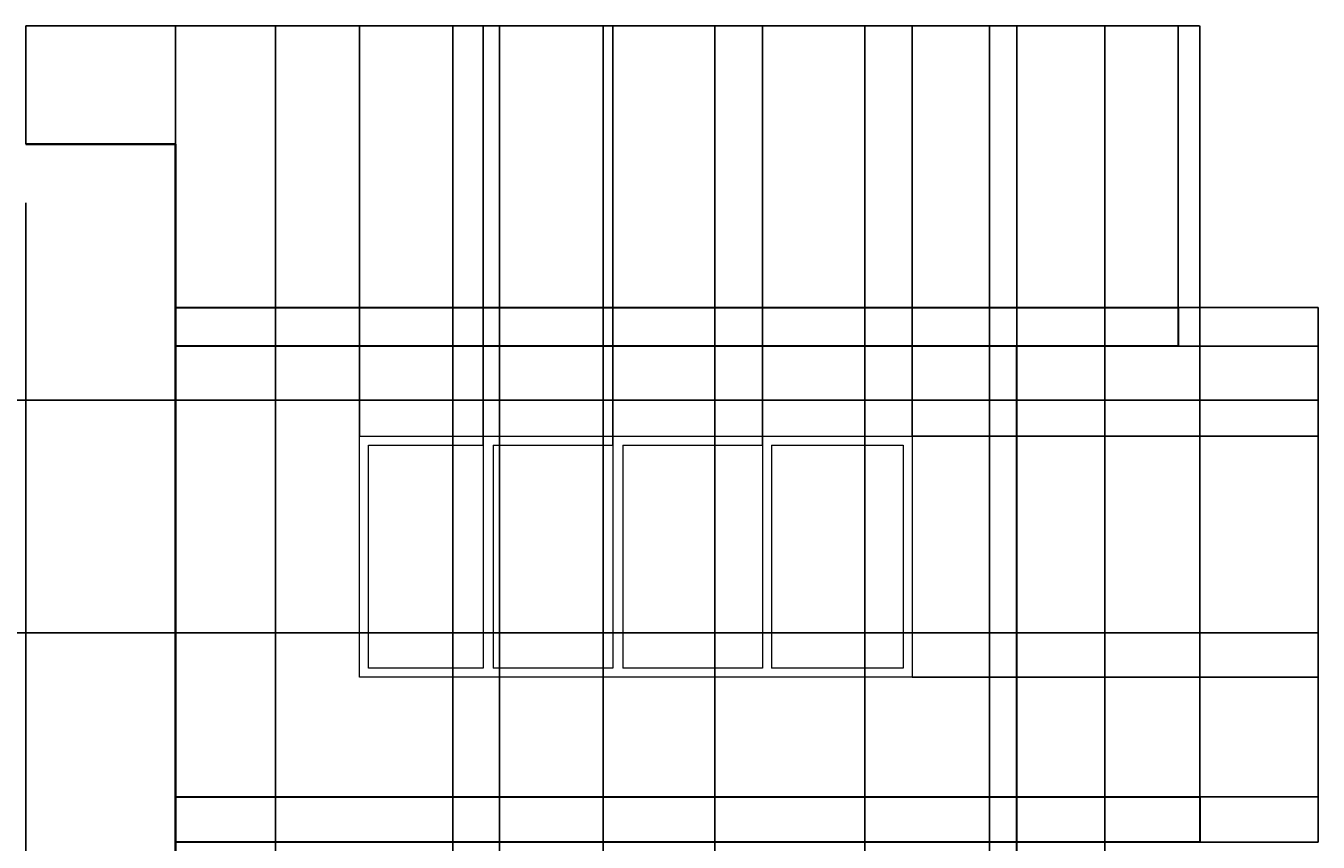
# Model space of a CAD drawing. Units: millimetres. Extents: x 1225 to 9865, y 11 to 4912.
# Tile 4 of 4: x 5562 to 9865, y 2192 to 4912. Entities that reach past the tile are written whole.
import ezdxf

# ---------------------------------------------------------------- set-up
doc = ezdxf.new("R2010")
doc.units = ezdxf.units.MM
for name, color, linetype, lineweight in [('A-ANNO-DIMS', 2, 'Continuous', 18), ('A-COLS', 7, 'Continuous', 35), ('A-FLOR', 7, 'Continuous', 30), ('A-GLAZ', 4, 'Continuous', 18), ('A-ROOF', 7, 'Continuous', 30), ('A-WALL', 7, 'Continuous', 30)]:
    doc.layers.add(name, color=color, linetype=linetype, lineweight=lineweight)
doc.styles.get("Standard").update_dxf_attribs({"font": 'arial.ttf'})
doc.dimstyles.get("Standard").update_dxf_attribs({"dimtxt": 0.18, "dimasz": 0.18, "dimexe": 0.18, "dimexo": 0.0625, "dimgap": 0.09, "dimtad": 0, "dimtih": 1, "dimtoh": 1, "dimdec": 4, "dimzin": 0, "dimdsep": 46, "dimtxsty": 'Standard', "dimcen": 0.09, "dimadec": 0, "dimazin": 0, "dimtfac": 1, "dimtdec": 4, "dimtofl": 0, "dimtmove": 0, "dimatfit": 3, "dimfxl": 1, "dimtolj": 1, "dimtzin": 0, "dimarcsym": 0})

# ---------------------------------------------------------------- blocks, each defined once
blk = doc.blocks.new('*D9')
at = {"layer": 'A-ANNO-DIMS', "color": 0, "lineweight": -2, "transparency": 16777216}
for p, q in [((5415.4, 4322.4), (5415.4, 10.6)), ((5561.8, 4322.4), (5561.8, 10.6)), ((5415.6, 10.8), (5488.1, 10.8)), ((5561.6, 10.8), (5489, 10.8))]:
    blk.add_line(p, q, dxfattribs=at)
at = {"layer": 'A-ANNO-DIMS', "color": 0, "transparency": 16777216}
for points in [[(5415.6, 10.8), (5415.6, 10.7), (5415.4, 10.8)], [(5561.6, 10.8), (5561.6, 10.7), (5561.8, 10.8)]]:
    blk.add_solid(points, dxfattribs=at)
at = {"layer": 'Defpoints', "color": 0, "transparency": 16777216}
for p in [(5415.4, 4322.4), (5561.8, 4322.4), (5561.8, 10.8)]:
    blk.add_point(p, dxfattribs=at)
at = {"layer": 'A-ANNO-DIMS', "color": 0, "transparency": 16777216, "insert": (5488.6, 10.8), "char_height": 0.18, "attachment_point": 5}
blk.add_mtext('\\A1;146.38', dxfattribs=at)
blk = doc.blocks.new('*D10')
at = {"layer": 'A-ANNO-DIMS', "color": 0, "lineweight": -2, "transparency": 16777216}
for p, q in [((5561.8, 4517.7), (5561.8, 4911.8)), ((5561.9, 4911.6), (5810.4, 4911.6)), ((6059.7, 4911.6), (5811.2, 4911.6)), ((6059.9, 4517.7), (6059.9, 4911.8))]:
    blk.add_line(p, q, dxfattribs=at)
at = {"layer": 'A-ANNO-DIMS', "color": 0, "transparency": 16777216}
for points in [[(5561.9, 4911.6), (5561.9, 4911.6), (5561.8, 4911.6)], [(6059.7, 4911.6), (6059.7, 4911.6), (6059.9, 4911.6)]]:
    blk.add_solid(points, dxfattribs=at)
at = {"layer": 'Defpoints', "color": 0, "transparency": 16777216}
for p in [(6059.9, 4911.6), (5561.8, 4517.6), (6059.9, 4517.6)]:
    blk.add_point(p, dxfattribs=at)
at = {"layer": 'A-ANNO-DIMS', "color": 0, "transparency": 16777216, "insert": (5810.8, 4911.6), "char_height": 0.18, "attachment_point": 5}
blk.add_mtext('\\A1;498.2', dxfattribs=at)
blk = doc.blocks.new('*D12')
at = {"layer": 'A-ANNO-DIMS', "color": 0, "lineweight": -2, "transparency": 16777216}
for p, q in [((6059.9, 496.3), (6059.9, 4911.8)), ((6060.1, 4911.6), (6226, 4911.6)), ((6392.9, 4911.6), (6226.9, 4911.6)), ((6393.1, 496.3), (6393.1, 4911.8))]:
    blk.add_line(p, q, dxfattribs=at)
at = {"layer": 'A-ANNO-DIMS', "color": 0, "transparency": 16777216}
for points in [[(6060.1, 4911.6), (6060.1, 4911.6), (6059.9, 4911.6)], [(6392.9, 4911.6), (6392.9, 4911.6), (6393.1, 4911.6)]]:
    blk.add_solid(points, dxfattribs=at)
at = {"layer": 'Defpoints', "color": 0, "transparency": 16777216}
for p in [(6393.1, 4911.6), (6059.9, 496.3), (6393.1, 496.3)]:
    blk.add_point(p, dxfattribs=at)
at = {"layer": 'A-ANNO-DIMS', "color": 0, "transparency": 16777216, "insert": (6226.5, 4911.6), "char_height": 0.18, "attachment_point": 5}
blk.add_mtext('\\A1;333.14', dxfattribs=at)
blk = doc.blocks.new('*D13')
at = {"layer": 'A-ANNO-DIMS', "color": 0, "lineweight": -2, "transparency": 16777216}
for p, q in [((6393.1, 1670.9), (6393.1, 4911.8)), ((6393.2, 4911.6), (6765.6, 4911.6)), ((7138.7, 4911.6), (6766.3, 4911.6)), ((7138.8, 1670.9), (7138.8, 4911.8))]:
    blk.add_line(p, q, dxfattribs=at)
at = {"layer": 'A-ANNO-DIMS', "color": 0, "transparency": 16777216}
for points in [[(6393.2, 4911.6), (6393.2, 4911.6), (6393.1, 4911.6)], [(7138.7, 4911.6), (7138.7, 4911.6), (7138.8, 4911.6)]]:
    blk.add_solid(points, dxfattribs=at)
at = {"layer": 'Defpoints', "color": 0, "transparency": 16777216}
for p in [(7138.8, 4911.6), (6393.1, 1670.8), (7138.8, 1670.8)]:
    blk.add_point(p, dxfattribs=at)
at = {"layer": 'A-ANNO-DIMS', "color": 0, "transparency": 16777216, "insert": (6765.9, 4911.6), "char_height": 0.18, "attachment_point": 5}
blk.add_mtext('\\A1;745.8', dxfattribs=at)
blk = doc.blocks.new('*D14')
at = {"layer": 'A-ANNO-DIMS', "color": 0, "lineweight": -2, "transparency": 16777216}
for p, q in [((6983.8, 1082), (6983.8, 4911.8)), ((6984, 4911.6), (7061.1, 4911.6)), ((7138.7, 4911.6), (7061.6, 4911.6)), ((7138.8, 496.3), (7138.8, 4911.8))]:
    blk.add_line(p, q, dxfattribs=at)
at = {"layer": 'A-ANNO-DIMS', "color": 0, "transparency": 16777216}
for points in [[(6984, 4911.6), (6984, 4911.6), (6983.8, 4911.6)], [(7138.7, 4911.6), (7138.7, 4911.6), (7138.8, 4911.6)]]:
    blk.add_solid(points, dxfattribs=at)
at = {"layer": 'Defpoints', "color": 0, "transparency": 16777216}
for p in [(7138.8, 4911.6), (6983.8, 1081.9), (7138.8, 496.3)]:
    blk.add_point(p, dxfattribs=at)
at = {"layer": 'A-ANNO-DIMS', "color": 0, "transparency": 16777216, "insert": (7061.3, 4911.6), "char_height": 0.18, "attachment_point": 5}
blk.add_mtext('\\A1;155', dxfattribs=at)
blk = doc.blocks.new('*D15')
at = {"layer": 'A-ANNO-DIMS', "color": 0, "lineweight": -2, "transparency": 16777216}
for p, q in [((7138.8, 1670.9), (7138.8, 4911.8)), ((7139, 4911.6), (7311.1, 4911.6)), ((7484.1, 4911.6), (7311.9, 4911.6)), ((7484.2, 1670.9), (7484.2, 4911.8))]:
    blk.add_line(p, q, dxfattribs=at)
at = {"layer": 'A-ANNO-DIMS', "color": 0, "transparency": 16777216}
for points in [[(7139, 4911.6), (7139, 4911.6), (7138.8, 4911.6)], [(7484.1, 4911.6), (7484.1, 4911.6), (7484.2, 4911.6)]]:
    blk.add_solid(points, dxfattribs=at)
at = {"layer": 'Defpoints', "color": 0, "transparency": 16777216}
for p in [(7484.2, 4911.6), (7138.8, 1670.8), (7484.2, 1670.8)]:
    blk.add_point(p, dxfattribs=at)
at = {"layer": 'A-ANNO-DIMS', "color": 0, "transparency": 16777216, "insert": (7311.5, 4911.6), "char_height": 0.18, "attachment_point": 5}
blk.add_mtext('\\A1;345.4', dxfattribs=at)
blk = doc.blocks.new('*D16')
at = {"layer": 'A-ANNO-DIMS', "color": 0, "lineweight": -2, "transparency": 16777216}
for p, q in [((8861.3, 496.3), (8861.3, 4911.8)), ((8861.4, 4911.6), (9007.3, 4911.6)), ((9153.9, 4911.6), (9008.1, 4911.6)), ((9154.1, 496.3), (9154.1, 4911.8))]:
    blk.add_line(p, q, dxfattribs=at)
at = {"layer": 'A-ANNO-DIMS', "color": 0, "transparency": 16777216}
for points in [[(8861.4, 4911.6), (8861.4, 4911.6), (8861.3, 4911.6)], [(9153.9, 4911.6), (9153.9, 4911.6), (9154.1, 4911.6)]]:
    blk.add_solid(points, dxfattribs=at)
at = {"layer": 'Defpoints', "color": 0, "transparency": 16777216}
for p in [(9154.1, 4911.6), (8861.3, 496.3), (9154.1, 496.3)]:
    blk.add_point(p, dxfattribs=at)
at = {"layer": 'A-ANNO-DIMS', "color": 0, "transparency": 16777216, "insert": (9007.7, 4911.6), "char_height": 0.18, "attachment_point": 5}
blk.add_mtext('\\A1;292.8', dxfattribs=at)
blk = doc.blocks.new('*D17')
at = {"layer": 'A-ANNO-DIMS', "color": 0, "lineweight": -2, "transparency": 16777216}
for p, q in [((8861.3, 2343), (8861.3, 4911.8)), ((8861.4, 4911.6), (9165.5, 4911.6)), ((9470.1, 4911.6), (9166.1, 4911.6)), ((9470.3, 2343), (9470.3, 4911.8))]:
    blk.add_line(p, q, dxfattribs=at)
at = {"layer": 'A-ANNO-DIMS', "color": 0, "transparency": 16777216}
for points in [[(8861.4, 4911.6), (8861.4, 4911.6), (8861.3, 4911.6)], [(9470.1, 4911.6), (9470.1, 4911.6), (9470.3, 4911.6)]]:
    blk.add_solid(points, dxfattribs=at)
at = {"layer": 'Defpoints', "color": 0, "transparency": 16777216}
for p in [(9470.3, 4911.6), (8861.3, 2343), (9470.3, 2343)]:
    blk.add_point(p, dxfattribs=at)
at = {"layer": 'A-ANNO-DIMS', "color": 0, "transparency": 16777216, "insert": (9165.8, 4911.6), "char_height": 0.18, "attachment_point": 5}
blk.add_mtext('\\A1;609', dxfattribs=at)
blk = doc.blocks.new('*D19')
at = {"layer": 'A-ANNO-DIMS', "color": 0, "lineweight": -2, "transparency": 16777216}
for p, q in [((6059.9, 3973.7), (6059.9, 4911.8)), ((6060.1, 4911.6), (7460.1, 4911.6)), ((8861.1, 4911.6), (7461.1, 4911.6)), ((8861.3, 3844.5), (8861.3, 4911.8))]:
    blk.add_line(p, q, dxfattribs=at)
at = {"layer": 'A-ANNO-DIMS', "color": 0, "transparency": 16777216}
for points in [[(6060.1, 4911.6), (6060.1, 4911.6), (6059.9, 4911.6)], [(8861.1, 4911.6), (8861.1, 4911.6), (8861.3, 4911.6)]]:
    blk.add_solid(points, dxfattribs=at)
at = {"layer": 'Defpoints', "color": 0, "transparency": 16777216}
for p in [(8861.3, 4911.6), (6059.9, 3973.7), (8861.3, 3844.4)]:
    blk.add_point(p, dxfattribs=at)
at = {"layer": 'A-ANNO-DIMS', "color": 0, "transparency": 16777216, "insert": (7460.6, 4911.6), "char_height": 0.18, "attachment_point": 5}
blk.add_mtext('\\A1;2801.3', dxfattribs=at)
blk = doc.blocks.new('*D20')
at = {"layer": 'A-ANNO-DIMS', "color": 0, "lineweight": -2, "transparency": 16777216}
for p, q in [((8861.3, 3844.5), (8861.3, 4911.8)), ((8861.4, 4911.6), (9129.2, 4911.6)), ((9397.8, 4911.6), (9130, 4911.6)), ((9398, 3973.7), (9398, 4911.8))]:
    blk.add_line(p, q, dxfattribs=at)
at = {"layer": 'A-ANNO-DIMS', "color": 0, "transparency": 16777216}
for points in [[(8861.4, 4911.6), (8861.4, 4911.6), (8861.3, 4911.6)], [(9397.8, 4911.6), (9397.8, 4911.6), (9398, 4911.6)]]:
    blk.add_solid(points, dxfattribs=at)
at = {"layer": 'Defpoints', "color": 0, "transparency": 16777216}
for p in [(9398, 4911.6), (9398, 3973.7), (8861.3, 3844.4)]:
    blk.add_point(p, dxfattribs=at)
at = {"layer": 'A-ANNO-DIMS', "color": 0, "transparency": 16777216, "insert": (9129.6, 4911.6), "char_height": 0.18, "attachment_point": 5}
blk.add_mtext('\\A1;536.7', dxfattribs=at)
blk = doc.blocks.new('*D25')
at = {"layer": 'A-ANNO-DIMS', "color": 0, "lineweight": -2, "transparency": 16777216}
for p, q in [((6059.9, 3844.5), (6059.9, 4911.8)), ((6060.1, 4911.6), (6365.9, 4911.6)), ((6672.4, 4911.6), (6366.7, 4911.6)), ((6672.6, 3545.1), (6672.6, 4911.8))]:
    blk.add_line(p, q, dxfattribs=at)
at = {"layer": 'A-ANNO-DIMS', "color": 0, "transparency": 16777216}
for points in [[(6060.1, 4911.6), (6060.1, 4911.6), (6059.9, 4911.6)], [(6672.4, 4911.6), (6672.4, 4911.6), (6672.6, 4911.6)]]:
    blk.add_solid(points, dxfattribs=at)
at = {"layer": 'Defpoints', "color": 0, "transparency": 16777216}
for p in [(6672.6, 4911.6), (6059.9, 3844.4), (6672.6, 3545)]:
    blk.add_point(p, dxfattribs=at)
at = {"layer": 'A-ANNO-DIMS', "color": 0, "transparency": 16777216, "insert": (6366.3, 4911.6), "char_height": 0.18, "attachment_point": 5}
blk.add_mtext('\\A1;612.7', dxfattribs=at)
blk = doc.blocks.new('*D30')
at = {"layer": 'A-ANNO-DIMS', "color": 0, "lineweight": -2, "transparency": 16777216}
for p, q in [((9470.3, 2343), (9864.4, 2343)), ((9864.3, 2342.8), (9864.3, 2267.8)), ((9864.3, 2192.3), (9864.3, 2267.4)), ((9470.3, 2192.2), (9864.4, 2192.2))]:
    blk.add_line(p, q, dxfattribs=at)
at = {"layer": 'A-ANNO-DIMS', "color": 0, "transparency": 16777216}
for points in [[(9864.2, 2342.8), (9864.3, 2342.8), (9864.3, 2343)], [(9864.2, 2192.3), (9864.3, 2192.3), (9864.3, 2192.2)]]:
    blk.add_solid(points, dxfattribs=at)
at = {"layer": 'Defpoints', "color": 0, "transparency": 16777216}
for p in [(9470.3, 2343), (9864.3, 2343), (9470.3, 2192.2)]:
    blk.add_point(p, dxfattribs=at)
at = {"layer": 'A-ANNO-DIMS', "color": 0, "transparency": 16777216, "insert": (9864.3, 2267.6), "char_height": 0.18, "attachment_point": 5}
blk.add_mtext('\\A1;150.8', dxfattribs=at)
blk = doc.blocks.new('*D37')
at = {"layer": 'A-ANNO-DIMS', "color": 0, "lineweight": -2, "transparency": 16777216}
for p, q in [((4669, 3664.7), (9864.4, 3664.7)), ((9864.3, 3664.5), (9864.3, 3277.4)), ((9864.3, 2889.9), (9864.3, 3277)), ((4669, 2889.7), (9864.4, 2889.7))]:
    blk.add_line(p, q, dxfattribs=at)
at = {"layer": 'A-ANNO-DIMS', "color": 0, "transparency": 16777216}
for points in [[(9864.2, 3664.5), (9864.3, 3664.5), (9864.3, 3664.7)], [(9864.2, 2889.9), (9864.3, 2889.9), (9864.3, 2889.7)]]:
    blk.add_solid(points, dxfattribs=at)
at = {"layer": 'Defpoints', "color": 0, "transparency": 16777216}
for p in [(4668.9, 3664.7), (9864.3, 3664.7), (4668.9, 2889.7)]:
    blk.add_point(p, dxfattribs=at)
at = {"layer": 'A-ANNO-DIMS', "color": 0, "transparency": 16777216, "insert": (9864.3, 3277.2), "char_height": 0.18, "attachment_point": 5}
blk.add_mtext('\\A1;775', dxfattribs=at)
blk = doc.blocks.new('*D40')
at = {"layer": 'A-ANNO-DIMS', "color": 0, "lineweight": -2, "transparency": 16777216}
for p, q in [((8512.8, 3545), (9864.4, 3545)), ((9864.3, 3544.8), (9864.3, 3143.4)), ((9864.3, 2741.6), (9864.3, 3143)), ((8512.8, 2741.4), (9864.4, 2741.4))]:
    blk.add_line(p, q, dxfattribs=at)
at = {"layer": 'A-ANNO-DIMS', "color": 0, "transparency": 16777216}
for points in [[(9864.2, 3544.8), (9864.3, 3544.8), (9864.3, 3545)], [(9864.2, 2741.6), (9864.3, 2741.6), (9864.3, 2741.4)]]:
    blk.add_solid(points, dxfattribs=at)
at = {"layer": 'Defpoints', "color": 0, "transparency": 16777216}
for p in [(8512.7, 3545), (9864.3, 3545), (8512.7, 2741.4)]:
    blk.add_point(p, dxfattribs=at)
at = {"layer": 'A-ANNO-DIMS', "color": 0, "transparency": 16777216, "insert": (9864.3, 3143.2), "char_height": 0.18, "attachment_point": 5}
blk.add_mtext('\\A1;803.6', dxfattribs=at)
blk = doc.blocks.new('*D41')
at = {"layer": 'A-ANNO-DIMS', "color": 0, "lineweight": -2, "transparency": 16777216}
for p, q in [((8512.8, 2741.4), (9864.4, 2741.4)), ((9864.3, 2741.2), (9864.3, 2542.4)), ((9864.3, 2343.2), (9864.3, 2542)), ((9470.3, 2343), (9864.4, 2343))]:
    blk.add_line(p, q, dxfattribs=at)
at = {"layer": 'A-ANNO-DIMS', "color": 0, "transparency": 16777216}
for points in [[(9864.2, 2741.2), (9864.3, 2741.2), (9864.3, 2741.4)], [(9864.2, 2343.2), (9864.3, 2343.2), (9864.3, 2343)]]:
    blk.add_solid(points, dxfattribs=at)
at = {"layer": 'Defpoints', "color": 0, "transparency": 16777216}
for p in [(8512.7, 2741.4), (9864.3, 2741.4), (9470.3, 2343)]:
    blk.add_point(p, dxfattribs=at)
at = {"layer": 'A-ANNO-DIMS', "color": 0, "transparency": 16777216, "insert": (9864.3, 2542.2), "char_height": 0.18, "attachment_point": 5}
blk.add_mtext('\\A1;398.4', dxfattribs=at)
blk = doc.blocks.new('*D42')
at = {"layer": 'A-ANNO-DIMS', "color": 0, "lineweight": -2, "transparency": 16777216}
for p, q in [((9398.1, 3844.4), (9864.4, 3844.4)), ((9864.3, 3844.3), (9864.3, 3694.9)), ((9864.3, 3545.2), (9864.3, 3694.5)), ((8512.8, 3545), (9864.4, 3545))]:
    blk.add_line(p, q, dxfattribs=at)
at = {"layer": 'A-ANNO-DIMS', "color": 0, "transparency": 16777216}
for points in [[(9864.2, 3844.3), (9864.3, 3844.3), (9864.3, 3844.4)], [(9864.2, 3545.2), (9864.3, 3545.2), (9864.3, 3545)]]:
    blk.add_solid(points, dxfattribs=at)
at = {"layer": 'Defpoints', "color": 0, "transparency": 16777216}
for p in [(9398, 3844.4), (9864.3, 3844.4), (8512.7, 3545)]:
    blk.add_point(p, dxfattribs=at)
at = {"layer": 'A-ANNO-DIMS', "color": 0, "transparency": 16777216, "insert": (9864.3, 3694.7), "char_height": 0.18, "attachment_point": 5}
blk.add_mtext('\\A1;299.4', dxfattribs=at)
blk = doc.blocks.new('*D43')
at = {"layer": 'A-ANNO-DIMS', "color": 0, "lineweight": -2, "transparency": 16777216}
for p, q in [((9398.1, 3973.7), (9864.4, 3973.7)), ((9864.3, 3973.5), (9864.3, 3909.2)), ((9864.3, 3844.6), (9864.3, 3908.9)), ((9398.1, 3844.4), (9864.4, 3844.4))]:
    blk.add_line(p, q, dxfattribs=at)
at = {"layer": 'A-ANNO-DIMS', "color": 0, "transparency": 16777216}
for points in [[(9864.2, 3973.5), (9864.3, 3973.5), (9864.3, 3973.7)], [(9864.2, 3844.6), (9864.3, 3844.6), (9864.3, 3844.4)]]:
    blk.add_solid(points, dxfattribs=at)
at = {"layer": 'Defpoints', "color": 0, "transparency": 16777216}
for p in [(9398, 3973.7), (9864.3, 3973.7), (9398, 3844.4)]:
    blk.add_point(p, dxfattribs=at)
at = {"layer": 'A-ANNO-DIMS', "color": 0, "transparency": 16777216, "insert": (9864.3, 3909), "char_height": 0.18, "attachment_point": 5}
blk.add_mtext('\\A1;129.22', dxfattribs=at)
blk = doc.blocks.new('*D48')
at = {"layer": 'A-ANNO-DIMS', "color": 0, "lineweight": -2, "transparency": 16777216}
for p, q in [((6672.6, 3545.1), (6672.6, 4911.8)), ((6672.8, 4911.6), (6878.3, 4911.6)), ((7084.4, 4911.6), (6878.9, 4911.6)), ((7084.6, 3515.1), (7084.6, 4911.8))]:
    blk.add_line(p, q, dxfattribs=at)
at = {"layer": 'A-ANNO-DIMS', "color": 0, "transparency": 16777216}
for points in [[(6672.8, 4911.6), (6672.8, 4911.6), (6672.6, 4911.6)], [(7084.4, 4911.6), (7084.4, 4911.6), (7084.6, 4911.6)]]:
    blk.add_solid(points, dxfattribs=at)
at = {"layer": 'Defpoints', "color": 0, "transparency": 16777216}
for p in [(7084.6, 4911.6), (6672.6, 3545), (7084.6, 3515)]:
    blk.add_point(p, dxfattribs=at)
at = {"layer": 'A-ANNO-DIMS', "color": 0, "transparency": 16777216, "insert": (6878.6, 4911.6), "char_height": 0.18, "attachment_point": 5}
blk.add_mtext('\\A1;412', dxfattribs=at)
blk = doc.blocks.new('*D49')
at = {"layer": 'A-ANNO-DIMS', "color": 0, "lineweight": -2, "transparency": 16777216}
for p, q in [((7084.6, 3515.1), (7084.6, 4911.8)), ((7084.8, 4911.6), (7300, 4911.6)), ((7516, 4911.6), (7300.8, 4911.6)), ((7516.2, 3515.1), (7516.2, 4911.8))]:
    blk.add_line(p, q, dxfattribs=at)
at = {"layer": 'A-ANNO-DIMS', "color": 0, "transparency": 16777216}
for points in [[(7084.8, 4911.6), (7084.8, 4911.6), (7084.6, 4911.6)], [(7516, 4911.6), (7516, 4911.6), (7516.2, 4911.6)]]:
    blk.add_solid(points, dxfattribs=at)
at = {"layer": 'Defpoints', "color": 0, "transparency": 16777216}
for p in [(7516.2, 4911.6), (7084.6, 3515), (7516.2, 3515)]:
    blk.add_point(p, dxfattribs=at)
at = {"layer": 'A-ANNO-DIMS', "color": 0, "transparency": 16777216, "insert": (7300.4, 4911.6), "char_height": 0.18, "attachment_point": 5}
blk.add_mtext('\\A1;431.6', dxfattribs=at)
blk = doc.blocks.new('*D50')
at = {"layer": 'A-ANNO-DIMS', "color": 0, "lineweight": -2, "transparency": 16777216}
for p, q in [((7516.2, 3515.1), (7516.2, 4911.8)), ((7516.3, 4911.6), (7764.9, 4911.6)), ((8014.3, 4911.6), (7765.7, 4911.6)), ((8014.4, 3515.1), (8014.4, 4911.8))]:
    blk.add_line(p, q, dxfattribs=at)
at = {"layer": 'A-ANNO-DIMS', "color": 0, "transparency": 16777216}
for points in [[(7516.3, 4911.6), (7516.3, 4911.6), (7516.2, 4911.6)], [(8014.3, 4911.6), (8014.3, 4911.6), (8014.4, 4911.6)]]:
    blk.add_solid(points, dxfattribs=at)
at = {"layer": 'Defpoints', "color": 0, "transparency": 16777216}
for p in [(8014.4, 4911.6), (7516.2, 3515), (8014.4, 3515)]:
    blk.add_point(p, dxfattribs=at)
at = {"layer": 'A-ANNO-DIMS', "color": 0, "transparency": 16777216, "insert": (7765.3, 4911.6), "char_height": 0.18, "attachment_point": 5}
blk.add_mtext('\\A1;498.3', dxfattribs=at)
blk = doc.blocks.new('*D51')
at = {"layer": 'A-ANNO-DIMS', "color": 0, "lineweight": -2, "transparency": 16777216}
for p, q in [((8014.4, 3515.1), (8014.4, 4911.8)), ((8014.6, 4911.6), (8263.2, 4911.6)), ((8512.6, 4911.6), (8264, 4911.6)), ((8512.7, 3545.1), (8512.7, 4911.8))]:
    blk.add_line(p, q, dxfattribs=at)
at = {"layer": 'A-ANNO-DIMS', "color": 0, "transparency": 16777216}
for points in [[(8014.6, 4911.6), (8014.6, 4911.6), (8014.4, 4911.6)], [(8512.6, 4911.6), (8512.6, 4911.6), (8512.7, 4911.6)]]:
    blk.add_solid(points, dxfattribs=at)
at = {"layer": 'Defpoints', "color": 0, "transparency": 16777216}
for p in [(8512.7, 4911.6), (8512.7, 3545), (8014.4, 3515)]:
    blk.add_point(p, dxfattribs=at)
at = {"layer": 'A-ANNO-DIMS', "color": 0, "transparency": 16777216, "insert": (8263.6, 4911.6), "char_height": 0.18, "attachment_point": 5}
blk.add_mtext('\\A1;498.3', dxfattribs=at)
blk = doc.blocks.new('*D52')
at = {"layer": 'A-ANNO-DIMS', "color": 0, "lineweight": -2, "transparency": 16777216}
for p, q in [((7484.2, 1670.9), (7484.2, 4911.8)), ((7484.4, 4911.6), (7670, 4911.6)), ((7856.1, 4911.6), (7670.5, 4911.6)), ((7856.2, 1640.9), (7856.2, 4911.8))]:
    blk.add_line(p, q, dxfattribs=at)
at = {"layer": 'A-ANNO-DIMS', "color": 0, "transparency": 16777216}
for points in [[(7484.4, 4911.6), (7484.4, 4911.6), (7484.2, 4911.6)], [(7856.1, 4911.6), (7856.1, 4911.6), (7856.2, 4911.6)]]:
    blk.add_solid(points, dxfattribs=at)
at = {"layer": 'Defpoints', "color": 0, "transparency": 16777216}
for p in [(7856.2, 4911.6), (7484.2, 1670.8), (7856.2, 1640.8)]:
    blk.add_point(p, dxfattribs=at)
at = {"layer": 'A-ANNO-DIMS', "color": 0, "transparency": 16777216, "insert": (7670.2, 4911.6), "char_height": 0.18, "attachment_point": 5}
blk.add_mtext('\\A1;372', dxfattribs=at)
blk = doc.blocks.new('*D53')
at = {"layer": 'A-ANNO-DIMS', "color": 0, "lineweight": -2, "transparency": 16777216}
for p, q in [((7856.2, 1640.9), (7856.2, 4911.8)), ((7856.4, 4911.6), (8105.4, 4911.6)), ((8355.2, 4911.6), (8106.2, 4911.6)), ((8355.4, 1640.9), (8355.4, 4911.8))]:
    blk.add_line(p, q, dxfattribs=at)
at = {"layer": 'A-ANNO-DIMS', "color": 0, "transparency": 16777216}
for points in [[(7856.4, 4911.6), (7856.4, 4911.6), (7856.2, 4911.6)], [(8355.2, 4911.6), (8355.2, 4911.6), (8355.4, 4911.6)]]:
    blk.add_solid(points, dxfattribs=at)
at = {"layer": 'Defpoints', "color": 0, "transparency": 16777216}
for p in [(8355.4, 4911.6), (7856.2, 1640.8), (8355.4, 1640.8)]:
    blk.add_point(p, dxfattribs=at)
at = {"layer": 'A-ANNO-DIMS', "color": 0, "transparency": 16777216, "insert": (8105.8, 4911.6), "char_height": 0.18, "attachment_point": 5}
blk.add_mtext('\\A1;499.1', dxfattribs=at)
blk = doc.blocks.new('*D54')
at = {"layer": 'A-ANNO-DIMS', "color": 0, "lineweight": -2, "transparency": 16777216}
for p, q in [((8355.4, 1640.9), (8355.4, 4911.8)), ((8355.5, 4911.6), (8562.6, 4911.6)), ((8770.5, 4911.6), (8563.5, 4911.6)), ((8770.7, 1670.9), (8770.7, 4911.8))]:
    blk.add_line(p, q, dxfattribs=at)
at = {"layer": 'A-ANNO-DIMS', "color": 0, "transparency": 16777216}
for points in [[(8355.5, 4911.6), (8355.5, 4911.6), (8355.4, 4911.6)], [(8770.5, 4911.6), (8770.5, 4911.6), (8770.7, 4911.6)]]:
    blk.add_solid(points, dxfattribs=at)
at = {"layer": 'Defpoints', "color": 0, "transparency": 16777216}
for p in [(8770.7, 4911.6), (8355.4, 1640.8), (8770.7, 1670.8)]:
    blk.add_point(p, dxfattribs=at)
at = {"layer": 'A-ANNO-DIMS', "color": 0, "transparency": 16777216, "insert": (8563, 4911.6), "char_height": 0.18, "attachment_point": 5}
blk.add_mtext('\\A1;415.36', dxfattribs=at)

msp = doc.modelspace()

# ---------------------------------------------------------------- linework, layer by layer
at = {"layer": 'A-COLS'}
for p, q in [((5561.752, 4517.596), (6059.917, 4517.596)), ((6059.917, 4517.596), (6059.917, 496.264))]:
    msp.add_line(p, q, dxfattribs=at)
at = {"layer": 'A-FLOR'}
for p, q in [((6059.917, 2342.982), (8861.261, 2342.982)), ((8861.261, 2342.982), (9470.268, 2342.982)), ((9470.268, 2342.982), (9470.268, 2192.169)), ((9470.268, 2192.169), (6059.917, 2192.169))]:
    msp.add_line(p, q, dxfattribs=at)
at = {"layer": 'A-GLAZ'}
for p, q in [((7084.577, 3515.013), (7084.577, 2771.387)), ((7117.576, 3515.013), (7117.576, 2771.387)), ((7516.162, 3515.013), (7516.162, 2771.387)), ((7550.024, 3515.013), (7550.024, 2771.387)), ((8014.447, 3515.013), (8014.447, 2771.387)), ((8044.511, 3515.013), (8044.511, 2771.387))]:
    msp.add_line(p, q, dxfattribs=at)
msp.add_lwpolyline([(6672.61, 3545.013), (8512.731, 3545.013), (8512.731, 2741.387), (6672.61, 2741.387)], close=True, dxfattribs=at)
for points in [[(7084.577, 2771.387), (6702.61, 2771.387), (6702.61, 3515.013), (7084.577, 3515.013)], [(7117.576, 3515.013), (7516.162, 3515.013)], [(7550.024, 3515.013), (8014.447, 3515.013)], [(8044.511, 3515.013), (8482.731, 3515.013), (8482.731, 2771.387), (8044.511, 2771.387)], [(7516.162, 2771.387), (7117.576, 2771.387)], [(8014.447, 2771.387), (7550.024, 2771.387)]]:
    msp.add_lwpolyline(points, dxfattribs=at)
at = {"layer": 'A-ROOF'}
for p, q in [((6059.917, 3844.439), (6059.917, 3973.656)), ((6059.917, 3973.656), (9397.988, 3973.656)), ((9397.988, 3973.656), (9397.988, 3844.439)), ((8861.261, 3844.439), (6059.917, 3844.439)), ((9397.988, 3844.439), (8861.261, 3844.439))]:
    msp.add_line(p, q, dxfattribs=at)
at = {"layer": 'A-WALL'}
msp.add_line((8861.261, 496.264), (8861.261, 3844.439), dxfattribs=at)

# ---------------------------------------------------------------- dimensions: what is measured, and where the dimension line sits
at = {"layer": 'A-ANNO-DIMS'}
for base, p1, p2, override, picture, middle in [((6059.917, 4911.596), (5561.752, 4517.596), (6059.917, 4517.596), {"dimdec": 1, "dimlfac": 1, "dimrnd": 0, "dimzin": 0, "dimdsep": 46, "dimlunit": 2}, '*D10', (5810.835, 4911.596)), ((6393.055, 4911.596), (6059.917, 496.264), (6393.055, 496.264), {"dimdec": 2, "dimlfac": 1, "dimrnd": 0, "dimzin": 0, "dimdsep": 46, "dimlunit": 2}, '*D12', (6226.486, 4911.596)), ((8861.261, 4911.596), (6059.917, 3973.656), (8861.261, 3844.439), {"dimdec": 1, "dimlfac": 1, "dimrnd": 0, "dimzin": 0, "dimdsep": 46, "dimlunit": 2}, '*D19', (7460.589, 4911.596)), ((6672.61, 4911.596), (6059.917, 3844.439), (6672.61, 3545.013), {"dimdec": 1, "dimlfac": 1, "dimrnd": 0, "dimzin": 0, "dimdsep": 46, "dimlunit": 2}, '*D25', (6366.263, 4911.596)), ((7138.844, 4911.596), (6393.055, 1670.836), (7138.844, 1670.836), {"dimdec": 1, "dimlfac": 1, "dimrnd": 0, "dimzin": 0, "dimdsep": 46, "dimlunit": 2}, '*D13', (6765.95, 4911.596)), ((7084.577, 4911.596), (6672.61, 3545.013), (7084.577, 3515.013), {"dimdec": 0, "dimlfac": 1, "dimrnd": 0, "dimzin": 0, "dimdsep": 46, "dimlunit": 2}, '*D48', (6878.594, 4911.596)), ((7138.844, 4911.596), (6983.847, 1081.944), (7138.844, 496.264), {"dimdec": 0, "dimlfac": 1, "dimrnd": 0, "dimzin": 0, "dimdsep": 46, "dimlunit": 2}, '*D14', (7061.346, 4911.596)), ((7516.162, 4911.596), (7084.577, 3515.013), (7516.162, 3515.013), {"dimdec": 1, "dimlfac": 1, "dimrnd": 0, "dimzin": 0, "dimdsep": 46, "dimlunit": 2}, '*D49', (7300.37, 4911.596)), ((7484.241, 4911.596), (7138.844, 1670.836), (7484.241, 1670.836), {"dimdec": 1, "dimlfac": 1, "dimrnd": 0, "dimzin": 0, "dimdsep": 46, "dimlunit": 2}, '*D15', (7311.543, 4911.596)), ((7856.234, 4911.596), (7484.241, 1670.836), (7856.234, 1640.836), {"dimdec": 0, "dimlfac": 1, "dimrnd": 0, "dimzin": 0, "dimdsep": 46, "dimlunit": 2}, '*D52', (7670.238, 4911.596)), ((8014.447, 4911.596), (7516.162, 3515.013), (8014.447, 3515.013), {"dimdec": 1, "dimlfac": 1, "dimrnd": 0, "dimzin": 0, "dimdsep": 46, "dimlunit": 2}, '*D50', (7765.305, 4911.596)), ((8355.362, 4911.596), (7856.234, 1640.836), (8355.362, 1640.836), {"dimdec": 1, "dimlfac": 1, "dimrnd": 0, "dimzin": 0, "dimdsep": 46, "dimlunit": 2}, '*D53', (8105.798, 4911.596)), ((8512.731, 4911.596), (8014.447, 3515.013), (8512.731, 3545.013), {"dimdec": 1, "dimlfac": 1, "dimrnd": 0, "dimzin": 0, "dimdsep": 46, "dimlunit": 2}, '*D51', (8263.589, 4911.596)), ((8770.718, 4911.596), (8355.362, 1640.836), (8770.718, 1670.836), {"dimdec": 2, "dimlfac": 1, "dimrnd": 0, "dimzin": 0, "dimdsep": 46, "dimlunit": 2}, '*D54', (8563.04, 4911.596)), ((9154.083, 4911.596), (8861.261, 496.264), (9154.083, 496.264), {"dimdec": 1, "dimlfac": 1, "dimrnd": 0, "dimzin": 0, "dimdsep": 46, "dimlunit": 2}, '*D16', (9007.672, 4911.596)), ((9470.268, 4911.596), (8861.261, 2342.982), (9470.268, 2342.982), {"dimdec": 0, "dimlfac": 1, "dimrnd": 0, "dimzin": 0, "dimdsep": 46, "dimlunit": 2}, '*D17', (9165.765, 4911.596)), ((9397.988, 4911.596), (8861.261, 3844.439), (9397.988, 3973.656), {"dimdec": 1, "dimlfac": 1, "dimrnd": 0, "dimzin": 0, "dimdsep": 46, "dimlunit": 2}, '*D20', (9129.625, 4911.596)), ((5561.752, 10.75), (5415.376, 4322.413), (5561.752, 4322.413), {"dimdec": 2, "dimlfac": 1, "dimrnd": 0, "dimzin": 0, "dimdsep": 46, "dimlunit": 2}, '*D9', (5488.564, 10.75))]:
    dim = msp.add_linear_dim(base=base, p1=p1, p2=p2, dimstyle='Standard', override=override, dxfattribs=at)
    dim.commit()
    dim.dimension.update_dxf_attribs({"geometry": picture, "text_midpoint": middle})
for base, p1, p2, override, picture, middle in [((9864.268, 3973.656), (9397.988, 3844.439), (9397.988, 3973.656), {"dimdec": 2, "dimlfac": 1, "dimrnd": 0, "dimzin": 0, "dimdsep": 46, "dimlunit": 2}, '*D43', (9864.268, 3909.047)), ((9864.268, 3844.439), (8512.731, 3545.013), (9397.988, 3844.439), {"dimdec": 1, "dimlfac": 1, "dimrnd": 0, "dimzin": 0, "dimdsep": 46, "dimlunit": 2}, '*D42', (9864.268, 3694.726)), ((9864.268, 3664.662), (4668.935, 2889.682), (4668.935, 3664.662), {"dimdec": 0, "dimlfac": 1, "dimrnd": 0, "dimzin": 0, "dimdsep": 46, "dimlunit": 2}, '*D37', (9864.268, 3277.172)), ((9864.268, 3545.013), (8512.731, 2741.387), (8512.731, 3545.013), {"dimdec": 1, "dimlfac": 1, "dimrnd": 0, "dimzin": 0, "dimdsep": 46, "dimlunit": 2}, '*D40', (9864.268, 3143.2)), ((9864.268, 2741.387), (9470.268, 2342.982), (8512.731, 2741.387), {"dimdec": 1, "dimlfac": 1, "dimrnd": 0, "dimzin": 0, "dimdsep": 46, "dimlunit": 2}, '*D41', (9864.268, 2542.185)), ((9864.268, 2342.982), (9470.268, 2192.169), (9470.268, 2342.982), {"dimdec": 1, "dimlfac": 1, "dimrnd": 0, "dimzin": 0, "dimdsep": 46, "dimlunit": 2}, '*D30', (9864.268, 2267.576))]:
    dim = msp.add_linear_dim(base=base, p1=p1, p2=p2, angle=90, dimstyle='Standard', override=override, dxfattribs=at)
    dim.commit()
    dim.dimension.update_dxf_attribs({"geometry": picture, "text_midpoint": middle})

doc.saveas('drawing.dxf')
